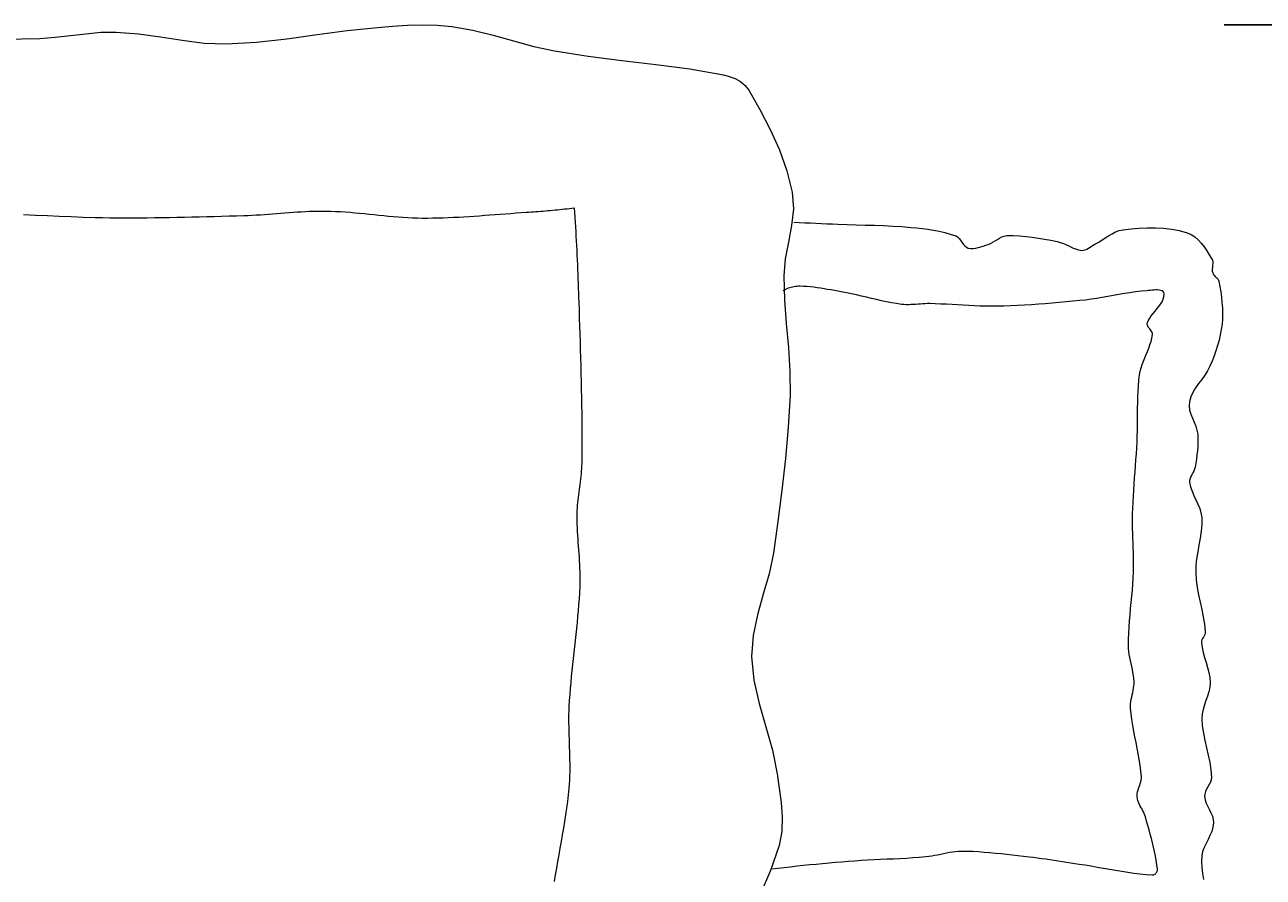
# Model space of a CAD drawing. Units: inches. Extents: x -15 to 423, y -713 to 71.
# Tile 22 of 24: x 311 to 364, y -137 to -101. Entities that reach past the tile are written whole.
import ezdxf

# ---------------------------------------------------------------- set-up
doc = ezdxf.new("R2010")
doc.units = ezdxf.units.IN
doc.header["$MEASUREMENT"] = 0
doc.layers.add('A-ANNO-DIMS', color=2, linetype='Continuous', lineweight=18)
doc.layers.add('A-FURN', color=9, linetype='Continuous', lineweight=13)
doc.styles.get("Standard").update_dxf_attribs({"font": 'arial.ttf'})
doc.dimstyles.get("Standard").update_dxf_attribs({"dimtxt": 0.18, "dimasz": 0.18, "dimexe": 0.18, "dimexo": 0.0625, "dimgap": 0.09, "dimtad": 0, "dimtih": 1, "dimtoh": 1, "dimdec": 0, "dimzin": 0, "dimdsep": 46, "dimlunit": 3, "dimtxsty": 'Standard', "dimcen": 0.09, "dimadec": 0, "dimazin": 0, "dimtfac": 1, "dimtdec": 0, "dimtofl": 0, "dimtmove": 0, "dimatfit": 3, "dimfxl": 1, "dimtolj": 1, "dimtzin": 0, "dimarcsym": 0})

# ---------------------------------------------------------------- blocks, each defined once
blk = doc.blocks.new('BED-DOUBLE')
for p, q in [((50.909, 70.114), (51.556, 70.189)), ((51.556, 70.189), (52.201, 70.268)), ((52.201, 70.268), (52.847, 70.326)), ((52.847, 70.326), (53.495, 70.339)), ((53.495, 70.339), (54.428, 70.266)), ((54.428, 70.266), (55.357, 70.134)), ((60.707, 70.052), (61.983, 70.229)), ((61.983, 70.229), (63.259, 70.403)), ((63.259, 70.403), (64.539, 70.536)), ((64.539, 70.536), (65.168, 70.585)), ((65.168, 70.585), (65.8, 70.625)), ((65.8, 70.625), (66.431, 70.645)), ((66.431, 70.645), (67.061, 70.633)), ((67.061, 70.633), (67.688, 70.576)), ((67.688, 70.576), (68.563, 70.418)), ((68.563, 70.418), (69.426, 70.201)), ((69.426, 70.201), (70.285, 69.959)), ((48.737, 70.043), (50.262, 70.068)), ((50.262, 70.068), (50.909, 70.114)), ((55.357, 70.134), (56.285, 69.988)), ((56.285, 69.988), (57.214, 69.874)), ((57.214, 69.874), (58.147, 69.837)), ((58.147, 69.837), (59.429, 69.908)), ((59.429, 69.908), (60.707, 70.052)), ((70.285, 69.959), (71.146, 69.727)), ((71.146, 69.727), (72.016, 69.538)), ((72.016, 69.538), (73.443, 69.316)), ((73.443, 69.316), (74.876, 69.137)), ((74.876, 69.137), (76.311, 68.967)), ((76.311, 68.967), (77.741, 68.775)), ((77.741, 68.775), (79.163, 68.528)), ((79.163, 68.528), (79.412, 68.464)), ((79.412, 68.464), (79.657, 68.368)), ((79.657, 68.368), (79.885, 68.24)), ((79.885, 68.24), (80.082, 68.078)), ((80.082, 68.078), (80.236, 67.88)), ((80.236, 67.88), (80.703, 67.06)), ((80.703, 67.06), (81.141, 66.219)), ((81.141, 66.219), (81.529, 65.356)), ((81.529, 65.356), (81.847, 64.47)), ((81.847, 64.47), (82.074, 63.56)), ((82.074, 63.56), (82.122, 62.86)), ((72.249, 62.834), (72.35, 62.845)), ((72.35, 62.845), (72.451, 62.855)), ((72.451, 62.855), (72.552, 62.866)), ((72.552, 62.866), (72.653, 62.877)), ((72.653, 62.877), (72.754, 62.888)), ((72.754, 62.888), (72.855, 62.9)), ((72.855, 62.9), (72.869, 62.701)), ((82.122, 62.86), (82.046, 62.156)), ((49.571, 62.62), (50.075, 62.595)), ((50.075, 62.595), (50.579, 62.572)), ((50.579, 62.572), (51.083, 62.55)), ((51.083, 62.55), (51.586, 62.53)), ((51.586, 62.53), (52.09, 62.513)), ((52.09, 62.513), (52.595, 62.499)), ((52.595, 62.499), (52.909, 62.492)), ((52.909, 62.492), (53.224, 62.487)), ((53.224, 62.487), (53.539, 62.483)), ((53.539, 62.483), (53.854, 62.481)), ((53.854, 62.481), (54.169, 62.481)), ((54.169, 62.481), (54.484, 62.482)), ((54.484, 62.482), (54.799, 62.484)), ((54.799, 62.484), (55.114, 62.488)), ((55.114, 62.488), (55.429, 62.492)), ((55.429, 62.492), (55.744, 62.497)), ((55.744, 62.497), (56.059, 62.504)), ((56.059, 62.504), (56.374, 62.511)), ((56.374, 62.511), (56.689, 62.518)), ((56.689, 62.518), (57.004, 62.526)), ((57.004, 62.526), (57.319, 62.535)), ((57.319, 62.535), (57.634, 62.543)), ((57.634, 62.543), (57.949, 62.552)), ((57.949, 62.552), (58.264, 62.561)), ((58.264, 62.561), (58.579, 62.57)), ((58.579, 62.57), (58.893, 62.579)), ((58.893, 62.579), (59.067, 62.585)), ((59.067, 62.585), (59.24, 62.592)), ((59.24, 62.592), (59.413, 62.602)), ((59.413, 62.602), (59.587, 62.612)), ((59.587, 62.612), (59.76, 62.624)), ((59.76, 62.624), (59.933, 62.637)), ((59.933, 62.637), (60.106, 62.65)), ((60.106, 62.65), (60.279, 62.663)), ((60.279, 62.663), (60.452, 62.677)), ((60.452, 62.677), (60.625, 62.691)), ((60.625, 62.691), (60.798, 62.704)), ((60.798, 62.704), (60.971, 62.717)), ((60.971, 62.717), (61.145, 62.729)), ((61.145, 62.729), (61.318, 62.739)), ((61.318, 62.739), (61.491, 62.749)), ((61.491, 62.749), (61.664, 62.756)), ((61.664, 62.756), (61.837, 62.762)), ((61.837, 62.762), (62.011, 62.766)), ((62.011, 62.766), (62.184, 62.768)), ((62.184, 62.768), (62.357, 62.767)), ((62.357, 62.767), (62.562, 62.762)), ((62.562, 62.762), (62.766, 62.754)), ((62.766, 62.754), (62.969, 62.743)), ((62.969, 62.743), (63.173, 62.73)), ((63.173, 62.73), (63.377, 62.714)), ((63.377, 62.714), (63.58, 62.696)), ((63.58, 62.696), (63.784, 62.677)), ((63.784, 62.677), (63.988, 62.657)), ((63.988, 62.657), (64.191, 62.637)), ((64.191, 62.637), (64.394, 62.616)), ((64.394, 62.616), (64.598, 62.595)), ((64.598, 62.595), (64.801, 62.574)), ((64.801, 62.574), (65.005, 62.555)), ((65.005, 62.555), (65.208, 62.537)), ((65.208, 62.537), (65.412, 62.52)), ((65.412, 62.52), (65.616, 62.505)), ((65.616, 62.505), (65.819, 62.493)), ((65.819, 62.493), (66.023, 62.483)), ((66.023, 62.483), (66.227, 62.476)), ((66.227, 62.476), (66.432, 62.473)), ((66.432, 62.473), (66.652, 62.473)), ((66.652, 62.473), (66.872, 62.475)), ((66.872, 62.475), (67.092, 62.479)), ((67.092, 62.479), (67.312, 62.486)), ((67.312, 62.486), (67.532, 62.494)), ((67.532, 62.494), (67.752, 62.503)), ((67.752, 62.503), (67.972, 62.514)), ((67.972, 62.514), (68.192, 62.527)), ((68.192, 62.527), (68.412, 62.54)), ((68.412, 62.54), (68.632, 62.555)), ((68.632, 62.555), (68.852, 62.57)), ((68.852, 62.57), (69.072, 62.586)), ((69.072, 62.586), (69.291, 62.602)), ((69.291, 62.602), (69.511, 62.619)), ((69.511, 62.619), (69.731, 62.636)), ((69.731, 62.636), (69.951, 62.652)), ((69.951, 62.652), (70.17, 62.669)), ((70.17, 62.669), (70.39, 62.685)), ((70.39, 62.685), (70.61, 62.701)), ((70.61, 62.701), (70.83, 62.716)), ((70.83, 62.716), (70.931, 62.723)), ((70.931, 62.723), (71.033, 62.73)), ((71.033, 62.73), (71.134, 62.737)), ((71.134, 62.737), (71.236, 62.745)), ((71.236, 62.745), (71.337, 62.753)), ((71.337, 62.753), (71.438, 62.761)), ((71.438, 62.761), (71.54, 62.769)), ((71.54, 62.769), (71.641, 62.778)), ((71.641, 62.778), (71.742, 62.787)), ((71.742, 62.787), (71.844, 62.796)), ((71.844, 62.796), (71.945, 62.805)), ((71.945, 62.805), (72.046, 62.814)), ((72.046, 62.814), (72.147, 62.824)), ((72.147, 62.824), (72.249, 62.834)), ((72.869, 62.701), (72.882, 62.501)), ((72.882, 62.501), (72.894, 62.302)), ((72.894, 62.302), (72.906, 62.103)), ((72.906, 62.103), (72.918, 61.903)), ((72.918, 61.903), (72.929, 61.704)), ((82.046, 62.156), (81.91, 61.449)), ((82.14, 62.295), (82.373, 62.284)), ((82.373, 62.284), (82.606, 62.273)), ((82.606, 62.273), (82.839, 62.263)), ((82.839, 62.263), (83.072, 62.252)), ((83.072, 62.252), (83.305, 62.242)), ((83.305, 62.242), (83.538, 62.231)), ((83.538, 62.231), (83.771, 62.221)), ((83.771, 62.221), (84.004, 62.21)), ((84.004, 62.21), (84.39, 62.196)), ((84.39, 62.196), (84.776, 62.185)), ((84.776, 62.185), (85.163, 62.175)), ((85.163, 62.175), (85.549, 62.165)), ((85.549, 62.165), (85.935, 62.152)), ((85.935, 62.152), (86.321, 62.134)), ((86.321, 62.134), (86.706, 62.11)), ((86.706, 62.11), (87.091, 62.077)), ((87.091, 62.077), (87.331, 62.053)), ((87.331, 62.053), (87.572, 62.025)), ((87.572, 62.025), (87.812, 61.994)), ((87.812, 61.994), (88.052, 61.957)), ((88.052, 61.957), (88.29, 61.912)), ((88.29, 61.912), (88.525, 61.859)), ((88.525, 61.859), (88.758, 61.795)), ((88.758, 61.795), (88.987, 61.72)), ((95.451, 61.723), (95.598, 61.81)), ((95.598, 61.81), (95.748, 61.884)), ((95.748, 61.884), (95.904, 61.941)), ((95.904, 61.941), (96.067, 61.975)), ((96.067, 61.975), (96.405, 62.013)), ((96.405, 62.013), (96.745, 62.042)), ((96.745, 62.042), (97.088, 62.058)), ((97.088, 62.058), (97.43, 62.06)), ((97.43, 62.06), (97.771, 62.042)), ((97.771, 62.042), (98.108, 62.004)), ((98.108, 62.004), (98.441, 61.941)), ((98.441, 61.941), (98.766, 61.851)), ((98.766, 61.851), (98.937, 61.777)), ((72.929, 61.704), (72.94, 61.505)), ((72.94, 61.505), (72.951, 61.305)), ((72.951, 61.305), (72.961, 61.106)), ((81.91, 61.449), (81.779, 60.741)), ((88.987, 61.72), (89.067, 61.676)), ((89.067, 61.676), (89.134, 61.612)), ((89.134, 61.612), (89.194, 61.536)), ((89.194, 61.536), (89.25, 61.453)), ((89.25, 61.453), (89.306, 61.371)), ((89.306, 61.371), (89.367, 61.298)), ((89.367, 61.298), (89.436, 61.239)), ((90.046, 61.25), (90.151, 61.285)), ((90.151, 61.285), (90.255, 61.321)), ((90.255, 61.321), (90.358, 61.356)), ((90.358, 61.356), (90.459, 61.397)), ((90.459, 61.397), (90.556, 61.45)), ((90.556, 61.45), (90.651, 61.509)), ((90.651, 61.509), (90.746, 61.57)), ((90.746, 61.57), (90.841, 61.627)), ((90.841, 61.627), (90.938, 61.675)), ((90.938, 61.675), (91.039, 61.71)), ((91.039, 61.71), (91.144, 61.726)), ((91.144, 61.726), (91.412, 61.729)), ((91.412, 61.729), (91.68, 61.719)), ((91.68, 61.719), (91.948, 61.697)), ((91.948, 61.697), (92.215, 61.665)), ((92.215, 61.665), (92.481, 61.626)), ((92.481, 61.626), (92.747, 61.58)), ((92.747, 61.58), (93.012, 61.531)), ((93.012, 61.531), (93.276, 61.479)), ((93.276, 61.479), (93.409, 61.444)), ((93.409, 61.444), (93.539, 61.395)), ((93.539, 61.395), (93.667, 61.337)), ((93.667, 61.337), (93.794, 61.275)), ((93.794, 61.275), (93.921, 61.216)), ((94.666, 61.238), (94.733, 61.282)), ((94.733, 61.282), (94.799, 61.325)), ((94.799, 61.325), (94.867, 61.363)), ((94.867, 61.363), (95.016, 61.444)), ((95.016, 61.444), (95.161, 61.535)), ((95.161, 61.535), (95.306, 61.63)), ((95.306, 61.63), (95.451, 61.723)), ((98.937, 61.777), (99.092, 61.674)), ((99.092, 61.674), (99.234, 61.548)), ((99.234, 61.548), (99.365, 61.405)), ((99.365, 61.405), (99.485, 61.248)), ((72.961, 61.106), (72.971, 60.906)), ((72.971, 60.906), (72.981, 60.707)), ((89.436, 61.239), (89.518, 61.202)), ((89.518, 61.202), (89.622, 61.184)), ((89.622, 61.184), (89.727, 61.183)), ((89.727, 61.183), (89.833, 61.195)), ((89.833, 61.195), (89.94, 61.219)), ((89.94, 61.219), (90.046, 61.25)), ((93.921, 61.216), (94.05, 61.164)), ((94.05, 61.164), (94.181, 61.125)), ((94.181, 61.125), (94.316, 61.104)), ((94.316, 61.104), (94.391, 61.107)), ((94.391, 61.107), (94.462, 61.126)), ((94.462, 61.126), (94.531, 61.156)), ((94.531, 61.156), (94.599, 61.194)), ((94.599, 61.194), (94.666, 61.238)), ((99.485, 61.248), (99.598, 61.085)), ((99.598, 61.085), (99.705, 60.919)), ((99.705, 60.919), (99.808, 60.757)), ((99.808, 60.757), (99.838, 60.69)), ((72.981, 60.707), (72.99, 60.507)), ((72.99, 60.507), (72.999, 60.308)), ((72.999, 60.308), (73.007, 60.108)), ((81.779, 60.741), (81.716, 60.031)), ((99.839, 60.384), (99.834, 60.305)), ((99.834, 60.305), (99.836, 60.227)), ((99.836, 60.227), (99.852, 60.153)), ((99.838, 60.69), (99.852, 60.618)), ((99.847, 60.463), (99.839, 60.384)), ((99.853, 60.542), (99.847, 60.463)), ((99.852, 60.618), (99.853, 60.542)), ((73.007, 60.108), (73.015, 59.909)), ((73.015, 59.909), (73.023, 59.709)), ((73.023, 59.709), (73.03, 59.51)), ((81.716, 60.031), (81.743, 59.019)), ((99.852, 60.153), (99.875, 60.104)), ((99.875, 60.104), (99.908, 60.059)), ((99.908, 60.059), (99.948, 60.017)), ((99.948, 60.017), (99.99, 59.977)), ((99.99, 59.977), (100.032, 59.936)), ((100.032, 59.936), (100.069, 59.894)), ((100.069, 59.894), (100.098, 59.848)), ((100.098, 59.848), (100.115, 59.797)), ((100.115, 59.797), (100.154, 59.573)), ((73.03, 59.51), (73.037, 59.31)), ((73.037, 59.31), (73.044, 59.111)), ((81.735, 59.422), (81.681, 59.391)), ((81.791, 59.451), (81.735, 59.422)), ((81.849, 59.477), (81.791, 59.451)), ((81.908, 59.5), (81.849, 59.477)), ((81.968, 59.521), (81.908, 59.5)), ((82.029, 59.539), (81.968, 59.521)), ((82.091, 59.554), (82.029, 59.539)), ((82.153, 59.567), (82.091, 59.554)), ((82.216, 59.576), (82.153, 59.567)), ((82.279, 59.583), (82.216, 59.576)), ((82.342, 59.586), (82.279, 59.583)), ((82.405, 59.587), (82.342, 59.586)), ((82.551, 59.582), (82.405, 59.587)), ((82.697, 59.573), (82.551, 59.582)), ((82.843, 59.56), (82.697, 59.573)), ((82.989, 59.544), (82.843, 59.56)), ((83.134, 59.525), (82.989, 59.544)), ((83.28, 59.503), (83.134, 59.525)), ((83.425, 59.48), (83.28, 59.503)), ((83.57, 59.455), (83.425, 59.48)), ((83.715, 59.429), (83.57, 59.455)), ((83.859, 59.403), (83.715, 59.429)), ((84.004, 59.376), (83.859, 59.403)), ((84.148, 59.35), (84.004, 59.376)), ((84.362, 59.31), (84.148, 59.35)), ((84.574, 59.266), (84.362, 59.31)), ((84.787, 59.219), (84.574, 59.266)), ((84.999, 59.171), (84.787, 59.219)), ((95.649, 59.195), (95.414, 59.154)), ((95.884, 59.236), (95.649, 59.195)), ((96.119, 59.275), (95.884, 59.236)), ((96.354, 59.312), (96.119, 59.275)), ((96.59, 59.345), (96.354, 59.312)), ((96.826, 59.373), (96.59, 59.345)), ((97.064, 59.395), (96.826, 59.373)), ((97.13, 59.401), (97.064, 59.395)), ((97.204, 59.409), (97.13, 59.401)), ((97.283, 59.417), (97.204, 59.409)), ((97.364, 59.424), (97.283, 59.417)), ((97.444, 59.429), (97.364, 59.424)), ((97.523, 59.429), (97.444, 59.429)), ((97.596, 59.423), (97.523, 59.429)), ((97.661, 59.411), (97.596, 59.423)), ((97.717, 59.389), (97.661, 59.411)), ((97.76, 59.358), (97.717, 59.389)), ((97.788, 59.316), (97.76, 59.358)), ((97.799, 59.261), (97.788, 59.316)), ((97.789, 59.144), (97.799, 59.261)), ((100.154, 59.573), (100.19, 59.348)), ((100.19, 59.348), (100.221, 59.121)), ((73.044, 59.111), (73.05, 58.911)), ((73.05, 58.911), (73.06, 58.576)), ((81.743, 59.019), (81.82, 58.007)), ((85.21, 59.121), (84.999, 59.171)), ((85.422, 59.072), (85.21, 59.121)), ((85.634, 59.023), (85.422, 59.072)), ((85.846, 58.976), (85.634, 59.023)), ((86.059, 58.931), (85.846, 58.976)), ((86.272, 58.89), (86.059, 58.931)), ((86.486, 58.853), (86.272, 58.89)), ((86.701, 58.821), (86.486, 58.853)), ((86.799, 58.811), (86.701, 58.821)), ((86.897, 58.806), (86.799, 58.811)), ((86.996, 58.805), (86.897, 58.806)), ((87.095, 58.808), (86.996, 58.805)), ((87.193, 58.813), (87.095, 58.808)), ((87.292, 58.819), (87.193, 58.813)), ((87.392, 58.827), (87.292, 58.819)), ((87.491, 58.835), (87.392, 58.827)), ((87.59, 58.842), (87.491, 58.835)), ((87.689, 58.848), (87.59, 58.842)), ((87.788, 58.851), (87.689, 58.848)), ((87.887, 58.851), (87.788, 58.851)), ((88.123, 58.845), (87.887, 58.851)), ((88.359, 58.835), (88.123, 58.845)), ((88.596, 58.824), (88.359, 58.835)), ((88.832, 58.81), (88.596, 58.824)), ((89.068, 58.797), (88.832, 58.81)), ((89.304, 58.783), (89.068, 58.797)), ((89.54, 58.77), (89.304, 58.783)), ((89.777, 58.758), (89.54, 58.77)), ((90.013, 58.749), (89.777, 58.758)), ((90.249, 58.743), (90.013, 58.749)), ((90.485, 58.741), (90.249, 58.743)), ((90.722, 58.743), (90.485, 58.741)), ((91.015, 58.75), (90.722, 58.743)), ((91.308, 58.76), (91.015, 58.75)), ((91.602, 58.773), (91.308, 58.76)), ((91.895, 58.788), (91.602, 58.773)), ((92.188, 58.805), (91.895, 58.788)), ((92.481, 58.824), (92.188, 58.805)), ((92.774, 58.846), (92.481, 58.824)), ((93.066, 58.869), (92.774, 58.846)), ((93.359, 58.894), (93.066, 58.869)), ((93.651, 58.921), (93.359, 58.894)), ((93.943, 58.949), (93.651, 58.921)), ((94.235, 58.978), (93.943, 58.949)), ((94.472, 59.005), (94.235, 58.978)), ((94.708, 59.038), (94.472, 59.005)), ((94.944, 59.074), (94.708, 59.038)), ((95.179, 59.113), (94.944, 59.074)), ((95.414, 59.154), (95.179, 59.113)), ((97.496, 58.631), (97.575, 58.728)), ((97.575, 58.728), (97.648, 58.827)), ((97.648, 58.827), (97.71, 58.929)), ((97.71, 58.929), (97.758, 59.034)), ((97.758, 59.034), (97.789, 59.144)), ((100.221, 59.121), (100.245, 58.894)), ((100.245, 58.894), (100.261, 58.667)), ((100.261, 58.667), (100.267, 58.439)), ((73.06, 58.576), (73.07, 58.24)), ((73.07, 58.24), (73.081, 57.905)), ((97.088, 58.015), (97.13, 58.127)), ((97.13, 58.127), (97.187, 58.233)), ((97.187, 58.233), (97.256, 58.336)), ((97.256, 58.336), (97.333, 58.436)), ((97.333, 58.436), (97.414, 58.534)), ((97.414, 58.534), (97.496, 58.631)), ((100.263, 58.213), (100.246, 57.986)), ((100.267, 58.439), (100.263, 58.213)), ((73.081, 57.905), (73.091, 57.57)), ((81.82, 58.007), (81.91, 56.995)), ((97.083, 57.974), (97.088, 58.015)), ((97.09, 57.934), (97.083, 57.974)), ((97.106, 57.895), (97.09, 57.934)), ((97.13, 57.856), (97.106, 57.895)), ((97.159, 57.818), (97.13, 57.856)), ((97.191, 57.78), (97.159, 57.818)), ((97.223, 57.743), (97.191, 57.78)), ((97.253, 57.704), (97.223, 57.743)), ((97.28, 57.666), (97.253, 57.704)), ((97.299, 57.626), (97.28, 57.666)), ((97.31, 57.585), (97.299, 57.626)), ((100.215, 57.758), (100.172, 57.53)), ((100.246, 57.986), (100.215, 57.758)), ((73.091, 57.57), (73.101, 57.234)), ((73.101, 57.234), (73.111, 56.899)), ((97.148, 56.972), (97.199, 57.112)), ((97.199, 57.112), (97.245, 57.254)), ((97.245, 57.254), (97.282, 57.397)), ((97.282, 57.397), (97.31, 57.543)), ((97.31, 57.543), (97.31, 57.585)), ((100.056, 57.082), (99.985, 56.861)), ((100.119, 57.305), (100.056, 57.082)), ((100.172, 57.53), (100.119, 57.305)), ((73.111, 56.899), (73.121, 56.563)), ((73.121, 56.563), (73.13, 56.228)), ((81.91, 56.995), (81.976, 55.984)), ((96.923, 56.417), (96.978, 56.556)), ((96.978, 56.556), (97.036, 56.695)), ((97.036, 56.695), (97.093, 56.833)), ((97.093, 56.833), (97.148, 56.972)), ((99.907, 56.642), (99.824, 56.425)), ((99.985, 56.861), (99.907, 56.642)), ((73.13, 56.228), (73.139, 55.893)), ((96.79, 55.992), (96.827, 56.135)), ((96.827, 56.135), (96.872, 56.276)), ((96.872, 56.276), (96.923, 56.417)), ((99.736, 56.211), (99.638, 56.015)), ((99.824, 56.425), (99.736, 56.211)), ((73.139, 55.893), (73.147, 55.557)), ((73.147, 55.557), (73.154, 55.222)), ((81.976, 55.984), (81.981, 54.972)), ((96.712, 55.377), (96.734, 55.611)), ((96.734, 55.611), (96.763, 55.846)), ((96.763, 55.846), (96.79, 55.992)), ((99.388, 55.647), (99.254, 55.467)), ((99.519, 55.828), (99.388, 55.647)), ((99.638, 56.015), (99.519, 55.828)), ((73.154, 55.222), (73.161, 54.886)), ((96.686, 54.905), (96.696, 55.141)), ((96.696, 55.141), (96.712, 55.377)), ((99.012, 55.1), (98.921, 54.904)), ((99.125, 55.286), (99.012, 55.1)), ((99.254, 55.467), (99.125, 55.286)), ((73.161, 54.886), (73.167, 54.551)), ((73.167, 54.551), (73.172, 54.215)), ((81.981, 54.972), (81.907, 53.633)), ((96.677, 54.432), (96.68, 54.668)), ((96.68, 54.668), (96.686, 54.905)), ((98.864, 54.697), (98.853, 54.524)), ((98.853, 54.524), (98.878, 54.353)), ((98.921, 54.904), (98.864, 54.697)), ((73.172, 54.215), (73.176, 53.88)), ((96.674, 53.721), (96.675, 53.958)), ((96.675, 54.195), (96.677, 54.432)), ((96.675, 53.958), (96.675, 54.195)), ((98.878, 54.353), (98.928, 54.183)), ((98.928, 54.183), (98.994, 54.014)), ((98.994, 54.014), (99.066, 53.845)), ((73.176, 53.88), (73.179, 53.545)), ((73.179, 53.545), (73.181, 53.209)), ((81.907, 53.633), (81.79, 52.296)), ((96.665, 53.247), (96.671, 53.484)), ((96.671, 53.484), (96.674, 53.721)), ((99.066, 53.845), (99.134, 53.674)), ((99.134, 53.674), (99.188, 53.502)), ((99.188, 53.502), (99.219, 53.328)), ((73.181, 53.209), (73.181, 52.874)), ((96.641, 52.755), (96.656, 53.011)), ((96.656, 53.011), (96.665, 53.247)), ((99.219, 53.328), (99.229, 53.153)), ((99.23, 52.978), (99.222, 52.803)), ((99.229, 53.153), (99.23, 52.978)), ((73.18, 52.538), (73.178, 52.203)), ((73.181, 52.874), (73.18, 52.538)), ((96.608, 52.244), (96.625, 52.5)), ((96.625, 52.5), (96.641, 52.755)), ((99.187, 52.453), (99.163, 52.278)), ((99.207, 52.628), (99.187, 52.453)), ((99.222, 52.803), (99.207, 52.628)), ((73.164, 51.87), (73.155, 51.76)), ((73.171, 51.981), (73.164, 51.87)), ((73.176, 52.092), (73.171, 51.981)), ((73.178, 52.203), (73.176, 52.092)), ((81.79, 52.296), (81.64, 50.963)), ((96.57, 51.734), (96.589, 51.989)), ((96.589, 51.989), (96.608, 52.244)), ((99.085, 51.849), (99.051, 51.769)), ((99.107, 51.931), (99.085, 51.849)), ((99.136, 52.104), (99.107, 51.931)), ((99.163, 52.278), (99.136, 52.104)), ((73.105, 51.318), (73.09, 51.208)), ((73.119, 51.428), (73.105, 51.318)), ((73.132, 51.539), (73.119, 51.428)), ((73.144, 51.649), (73.132, 51.539)), ((73.155, 51.76), (73.144, 51.649)), ((96.533, 51.223), (96.551, 51.478)), ((96.551, 51.478), (96.57, 51.734)), ((98.896, 51.458), (98.878, 51.378)), ((98.878, 51.378), (98.878, 51.295)), ((98.928, 51.536), (98.896, 51.458)), ((98.968, 51.614), (98.928, 51.536)), ((99.01, 51.691), (98.968, 51.614)), ((99.051, 51.769), (99.01, 51.691)), ((73.046, 50.877), (73.032, 50.767)), ((73.061, 50.987), (73.046, 50.877)), ((73.076, 51.098), (73.061, 50.987)), ((73.09, 51.208), (73.076, 51.098)), ((81.64, 50.963), (81.466, 49.632)), ((96.499, 50.712), (96.515, 50.968)), ((96.515, 50.968), (96.533, 51.223)), ((98.878, 51.295), (98.918, 51.103)), ((98.918, 51.103), (98.981, 50.917)), ((98.981, 50.917), (99.059, 50.733)), ((72.985, 50.325), (72.977, 50.214)), ((72.995, 50.435), (72.985, 50.325)), ((73.006, 50.546), (72.995, 50.435)), ((73.018, 50.656), (73.006, 50.546)), ((73.032, 50.767), (73.018, 50.656)), ((96.473, 50.201), (96.485, 50.456)), ((96.485, 50.456), (96.499, 50.712)), ((99.059, 50.733), (99.144, 50.552)), ((99.144, 50.552), (99.228, 50.37)), ((99.228, 50.37), (99.301, 50.186)), ((72.969, 49.992), (72.967, 49.837)), ((72.967, 49.837), (72.969, 49.681)), ((72.972, 50.103), (72.969, 49.992)), ((72.977, 50.214), (72.972, 50.103)), ((96.461, 49.743), (96.464, 49.945)), ((96.464, 49.945), (96.473, 50.201)), ((99.301, 50.186), (99.357, 49.999)), ((99.357, 49.999), (99.386, 49.806)), ((99.386, 49.806), (99.389, 49.514)), ((72.969, 49.681), (72.973, 49.525)), ((72.973, 49.525), (72.978, 49.37)), ((72.978, 49.37), (72.986, 49.214)), ((81.466, 49.632), (81.275, 48.303)), ((96.461, 49.54), (96.461, 49.743)), ((96.464, 49.337), (96.461, 49.54)), ((96.47, 49.135), (96.464, 49.337)), ((99.365, 49.224), (99.323, 48.933)), ((99.389, 49.514), (99.365, 49.224)), ((72.986, 49.214), (72.995, 49.058)), ((72.995, 49.058), (73.004, 48.903)), ((73.004, 48.903), (73.015, 48.747)), ((73.015, 48.747), (73.026, 48.591)), ((96.477, 48.932), (96.47, 49.135)), ((96.484, 48.73), (96.477, 48.932)), ((96.492, 48.527), (96.484, 48.73)), ((99.323, 48.933), (99.271, 48.643)), ((73.026, 48.591), (73.037, 48.436)), ((73.037, 48.436), (73.048, 48.28)), ((73.048, 48.28), (73.059, 48.125)), ((81.275, 48.303), (81.093, 47.426)), ((96.499, 48.325), (96.492, 48.527)), ((96.504, 48.122), (96.499, 48.325)), ((99.217, 48.353), (99.171, 48.063)), ((99.271, 48.643), (99.217, 48.353)), ((73.059, 48.125), (73.068, 47.969)), ((73.068, 47.969), (73.077, 47.813)), ((73.077, 47.813), (73.084, 47.658)), ((73.084, 47.658), (73.09, 47.502)), ((96.502, 47.515), (96.506, 47.717)), ((96.507, 47.92), (96.504, 48.122)), ((96.506, 47.717), (96.507, 47.92)), ((99.141, 47.772), (99.135, 47.48)), ((99.171, 48.063), (99.141, 47.772)), ((73.09, 47.502), (73.093, 47.347)), ((73.094, 47.191), (73.092, 47.035)), ((73.093, 47.347), (73.094, 47.191)), ((81.093, 47.426), (80.849, 46.558)), ((96.475, 46.994), (96.491, 47.254)), ((96.491, 47.254), (96.502, 47.515)), ((99.135, 47.48), (99.157, 47.165)), ((99.157, 47.165), (99.2, 46.852)), ((73.075, 46.626), (73.06, 46.373)), ((73.087, 46.88), (73.075, 46.626)), ((73.092, 47.035), (73.087, 46.88)), ((96.432, 46.473), (96.455, 46.733)), ((96.455, 46.733), (96.475, 46.994)), ((99.2, 46.852), (99.257, 46.541)), ((73.042, 46.119), (73.022, 45.866)), ((73.06, 46.373), (73.042, 46.119)), ((80.849, 46.558), (80.603, 45.691)), ((96.382, 45.953), (96.407, 46.213)), ((96.407, 46.213), (96.432, 46.473)), ((99.257, 46.541), (99.322, 46.23)), ((99.322, 46.23), (99.389, 45.92)), ((73, 45.613), (72.976, 45.36)), ((73.022, 45.866), (73, 45.613)), ((80.603, 45.691), (80.417, 44.818)), ((96.336, 45.433), (96.358, 45.693)), ((96.358, 45.693), (96.382, 45.953)), ((99.389, 45.92), (99.452, 45.609)), ((99.452, 45.609), (99.505, 45.296)), ((72.95, 45.107), (72.924, 44.854)), ((72.976, 45.36), (72.95, 45.107)), ((96.302, 44.912), (96.317, 45.173)), ((96.317, 45.173), (96.336, 45.433)), ((99.505, 45.296), (99.54, 44.982)), ((72.897, 44.601), (72.869, 44.349)), ((72.924, 44.854), (72.897, 44.601)), ((80.417, 44.818), (80.352, 43.933)), ((96.29, 44.391), (96.293, 44.652)), ((96.293, 44.652), (96.302, 44.912)), ((99.377, 44.58), (99.374, 44.52)), ((99.374, 44.52), (99.405, 44.305)), ((99.395, 44.638), (99.377, 44.58)), ((99.423, 44.695), (99.395, 44.638)), ((99.456, 44.751), (99.423, 44.695)), ((99.489, 44.807), (99.456, 44.751)), ((99.518, 44.864), (99.489, 44.807)), ((99.536, 44.922), (99.518, 44.864)), ((99.54, 44.982), (99.536, 44.922)), ((72.841, 44.096), (72.813, 43.843)), ((72.869, 44.349), (72.841, 44.096)), ((96.295, 44.263), (96.29, 44.391)), ((96.307, 44.136), (96.295, 44.263)), ((96.325, 44.009), (96.307, 44.136)), ((96.348, 43.882), (96.325, 44.009)), ((99.405, 44.305), (99.453, 44.092)), ((99.453, 44.092), (99.512, 43.881)), ((72.785, 43.591), (72.759, 43.338)), ((72.813, 43.843), (72.785, 43.591)), ((80.352, 43.933), (80.453, 42.928)), ((96.374, 43.756), (96.348, 43.882)), ((96.402, 43.63), (96.374, 43.756)), ((96.43, 43.504), (96.402, 43.63)), ((96.457, 43.378), (96.43, 43.504)), ((99.512, 43.881), (99.576, 43.671)), ((99.576, 43.671), (99.637, 43.46)), ((72.733, 43.085), (72.709, 42.832)), ((72.759, 43.338), (72.733, 43.085)), ((96.481, 43.251), (96.457, 43.378)), ((96.502, 43.124), (96.481, 43.251)), ((96.517, 42.997), (96.502, 43.124)), ((96.525, 42.869), (96.517, 42.997)), ((99.637, 43.46), (99.689, 43.249)), ((99.689, 43.249), (99.726, 43.036)), ((99.726, 43.036), (99.74, 42.82)), ((72.687, 42.579), (72.667, 42.325)), ((72.709, 42.832), (72.687, 42.579)), ((80.453, 42.928), (80.676, 41.938)), ((96.468, 42.4), (96.487, 42.494)), ((96.487, 42.494), (96.504, 42.587)), ((96.504, 42.587), (96.517, 42.681)), ((96.517, 42.681), (96.525, 42.775)), ((96.525, 42.775), (96.525, 42.869)), ((99.686, 42.439), (99.63, 42.252)), ((99.726, 42.628), (99.686, 42.439)), ((99.74, 42.82), (99.726, 42.628)), ((72.649, 42.072), (72.634, 41.818)), ((72.667, 42.325), (72.649, 42.072)), ((80.676, 41.938), (80.958, 40.954)), ((96.378, 41.839), (96.383, 41.933)), ((96.383, 41.933), (96.393, 42.027)), ((96.393, 42.027), (96.409, 42.12)), ((96.409, 42.12), (96.427, 42.214)), ((96.427, 42.214), (96.447, 42.307)), ((96.447, 42.307), (96.468, 42.4)), ((99.565, 42.066), (99.5, 41.88)), ((99.63, 42.252), (99.565, 42.066)), ((72.621, 41.473), (72.619, 41.3)), ((72.626, 41.646), (72.621, 41.473)), ((72.634, 41.818), (72.626, 41.646)), ((96.381, 41.746), (96.378, 41.839)), ((96.405, 41.502), (96.381, 41.746)), ((96.436, 41.259), (96.405, 41.502)), ((99.406, 41.504), (99.393, 41.313)), ((99.444, 41.693), (99.406, 41.504)), ((99.5, 41.88), (99.444, 41.693)), ((72.619, 41.3), (72.62, 41.127)), ((72.62, 41.127), (72.622, 40.954)), ((72.622, 40.954), (72.625, 40.78)), ((80.958, 40.954), (81.233, 39.968)), ((96.474, 41.016), (96.436, 41.259)), ((96.516, 40.775), (96.474, 41.016)), ((99.393, 41.313), (99.412, 40.998)), ((99.412, 40.998), (99.457, 40.685)), ((72.625, 40.78), (72.63, 40.607)), ((72.63, 40.607), (72.636, 40.434)), ((72.636, 40.434), (72.642, 40.261)), ((96.562, 40.533), (96.516, 40.775)), ((96.609, 40.292), (96.562, 40.533)), ((99.457, 40.685), (99.519, 40.374)), ((99.519, 40.374), (99.589, 40.064)), ((72.642, 40.261), (72.648, 40.088)), ((72.648, 40.088), (72.654, 39.914)), ((72.654, 39.914), (72.659, 39.741)), ((81.233, 39.968), (81.436, 38.971)), ((96.656, 40.051), (96.609, 40.292)), ((96.702, 39.81), (96.656, 40.051)), ((96.744, 39.568), (96.702, 39.81)), ((99.589, 40.064), (99.661, 39.753)), ((72.659, 39.741), (72.662, 39.568)), ((72.662, 39.568), (72.665, 39.395)), ((72.665, 39.395), (72.665, 39.222)), ((96.782, 39.326), (96.744, 39.568)), ((96.812, 39.083), (96.782, 39.326)), ((99.661, 39.753), (99.724, 39.442)), ((99.724, 39.442), (99.773, 39.13)), ((72.659, 38.877), (72.652, 38.704)), ((72.664, 39.049), (72.659, 38.877)), ((72.665, 39.222), (72.664, 39.049)), ((81.436, 38.971), (81.528, 38.364)), ((96.835, 38.839), (96.812, 39.083)), ((96.827, 38.695), (96.836, 38.767)), ((96.836, 38.767), (96.835, 38.839)), ((99.773, 39.13), (99.798, 38.815)), ((99.798, 38.815), (99.788, 38.71)), ((72.627, 38.359), (72.598, 38.076)), ((72.641, 38.531), (72.627, 38.359)), ((72.652, 38.704), (72.641, 38.531)), ((81.528, 38.364), (81.611, 37.75)), ((96.677, 38.202), (96.696, 38.272)), ((96.696, 38.272), (96.719, 38.343)), ((96.719, 38.343), (96.744, 38.413)), ((96.744, 38.413), (96.769, 38.483)), ((96.769, 38.483), (96.792, 38.554)), ((96.792, 38.554), (96.812, 38.624)), ((96.812, 38.624), (96.827, 38.695)), ((99.596, 38.312), (99.548, 38.213)), ((99.651, 38.41), (99.596, 38.312)), ((99.707, 38.509), (99.651, 38.41)), ((99.755, 38.608), (99.707, 38.509)), ((99.788, 38.71), (99.755, 38.608)), ((72.565, 37.793), (72.528, 37.51)), ((72.598, 38.076), (72.565, 37.793)), ((81.611, 37.75), (81.655, 37.136)), ((96.657, 38.06), (96.663, 38.131)), ((96.659, 37.988), (96.657, 38.06)), ((96.671, 37.913), (96.659, 37.988)), ((96.663, 38.131), (96.677, 38.202)), ((96.69, 37.84), (96.671, 37.913)), ((96.715, 37.769), (96.69, 37.84)), ((96.745, 37.699), (96.715, 37.769)), ((99.516, 38.111), (99.507, 38.006)), ((99.507, 38.006), (99.529, 37.861)), ((99.548, 38.213), (99.516, 38.111)), ((99.529, 37.861), (99.576, 37.721)), ((99.576, 37.721), (99.64, 37.583)), ((72.488, 37.228), (72.445, 36.947)), ((72.528, 37.51), (72.488, 37.228)), ((96.778, 37.63), (96.745, 37.699)), ((96.814, 37.562), (96.778, 37.63)), ((96.851, 37.494), (96.814, 37.562)), ((96.887, 37.425), (96.851, 37.494)), ((96.923, 37.357), (96.887, 37.425)), ((96.955, 37.287), (96.923, 37.357)), ((96.984, 37.216), (96.955, 37.287)), ((97.008, 37.144), (96.984, 37.216)), ((99.64, 37.583), (99.711, 37.447)), ((99.711, 37.447), (99.78, 37.311)), ((99.78, 37.311), (99.838, 37.174)), ((72.399, 36.665), (72.352, 36.384)), ((72.445, 36.947), (72.399, 36.665)), ((81.655, 37.136), (81.634, 36.529)), ((97.059, 36.962), (97.008, 37.144)), ((97.11, 36.78), (97.059, 36.962)), ((97.161, 36.597), (97.11, 36.78)), ((99.862, 36.708), (99.809, 36.534)), ((99.838, 37.174), (99.877, 37.034)), ((99.888, 36.889), (99.862, 36.708)), ((99.877, 37.034), (99.888, 36.889)), ((72.352, 36.384), (72.303, 36.103)), ((81.634, 36.529), (81.518, 35.937)), ((97.211, 36.414), (97.161, 36.597)), ((97.26, 36.231), (97.211, 36.414)), ((97.306, 36.048), (97.26, 36.231)), ((99.654, 36.194), (99.569, 36.025)), ((99.737, 36.363), (99.654, 36.194)), ((99.809, 36.534), (99.737, 36.363)), ((72.254, 35.822), (72.204, 35.541)), ((72.303, 36.103), (72.254, 35.822)), ((81.518, 35.937), (81.158, 34.884)), ((88.476, 35.6), (88.602, 35.626)), ((88.602, 35.626), (88.728, 35.65)), ((88.728, 35.65), (88.855, 35.67)), ((88.855, 35.67), (88.982, 35.686)), ((88.982, 35.686), (89.109, 35.697)), ((89.109, 35.697), (89.237, 35.7)), ((89.237, 35.7), (89.476, 35.697)), ((89.476, 35.697), (89.714, 35.689)), ((89.714, 35.689), (89.952, 35.676)), ((89.952, 35.676), (90.19, 35.659)), ((90.19, 35.659), (90.428, 35.639)), ((90.428, 35.639), (90.665, 35.617)), ((90.665, 35.617), (90.903, 35.592)), ((97.35, 35.864), (97.306, 36.048)), ((97.391, 35.68), (97.35, 35.864)), ((97.429, 35.494), (97.391, 35.68)), ((99.427, 35.681), (99.387, 35.502)), ((99.49, 35.855), (99.427, 35.681)), ((99.569, 36.025), (99.49, 35.855)), ((72.153, 35.261), (72.103, 34.98)), ((72.204, 35.541), (72.153, 35.261)), ((82.275, 35.069), (82.546, 35.098)), ((82.546, 35.098), (82.818, 35.125)), ((82.818, 35.125), (83.089, 35.152)), ((83.089, 35.152), (83.36, 35.178)), ((83.36, 35.178), (83.631, 35.203)), ((83.631, 35.203), (83.903, 35.227)), ((83.903, 35.227), (84.174, 35.251)), ((84.174, 35.251), (84.446, 35.273)), ((84.446, 35.273), (84.718, 35.293)), ((84.718, 35.293), (84.991, 35.311)), ((84.991, 35.311), (85.263, 35.326)), ((85.263, 35.326), (85.536, 35.34)), ((85.536, 35.34), (85.809, 35.353)), ((85.809, 35.353), (86.081, 35.365)), ((86.081, 35.365), (86.354, 35.378)), ((86.354, 35.378), (86.627, 35.392)), ((86.627, 35.392), (86.899, 35.406)), ((86.899, 35.406), (87.172, 35.423)), ((87.172, 35.423), (87.444, 35.443)), ((87.444, 35.443), (87.716, 35.465)), ((87.716, 35.465), (87.843, 35.479)), ((87.843, 35.479), (87.97, 35.499)), ((87.97, 35.499), (88.097, 35.521)), ((88.097, 35.521), (88.223, 35.547)), ((88.223, 35.547), (88.35, 35.573)), ((88.35, 35.573), (88.476, 35.6)), ((90.903, 35.592), (91.14, 35.565)), ((91.14, 35.565), (91.377, 35.538)), ((91.377, 35.538), (91.614, 35.51)), ((91.614, 35.51), (91.851, 35.483)), ((91.851, 35.483), (92.088, 35.456)), ((92.088, 35.456), (92.265, 35.436)), ((92.265, 35.436), (92.441, 35.414)), ((92.441, 35.414), (92.617, 35.39)), ((92.617, 35.39), (92.793, 35.365)), ((92.793, 35.365), (92.969, 35.34)), ((92.969, 35.34), (93.145, 35.314)), ((93.145, 35.314), (93.321, 35.287)), ((93.321, 35.287), (93.497, 35.259)), ((93.497, 35.259), (93.672, 35.232)), ((93.672, 35.232), (93.848, 35.205)), ((93.848, 35.205), (94.024, 35.178)), ((94.024, 35.178), (94.199, 35.152)), ((94.199, 35.152), (94.458, 35.112)), ((94.458, 35.112), (94.715, 35.069)), ((97.463, 35.309), (97.429, 35.494)), ((97.493, 35.122), (97.463, 35.309)), ((97.518, 34.935), (97.493, 35.122)), ((99.387, 35.502), (99.374, 35.255)), ((99.374, 35.255), (99.391, 35.004)), ((72.054, 34.699), (72.006, 34.418)), ((72.103, 34.98), (72.054, 34.699)), ((81.158, 34.884), (80.717, 33.859)), ((81.192, 34.944), (81.463, 34.976)), ((81.463, 34.976), (81.734, 35.008)), ((81.734, 35.008), (82.005, 35.039)), ((82.005, 35.039), (82.275, 35.069)), ((94.715, 35.069), (94.973, 35.025)), ((94.973, 35.025), (95.23, 34.979)), ((95.23, 34.979), (95.488, 34.933)), ((95.488, 34.933), (95.745, 34.888)), ((95.745, 34.888), (96.003, 34.845)), ((96.003, 34.845), (96.261, 34.805)), ((96.261, 34.805), (96.519, 34.768)), ((96.519, 34.768), (96.778, 34.735)), ((96.778, 34.735), (97.038, 34.708)), ((97.038, 34.708), (97.298, 34.688)), ((97.298, 34.688), (97.325, 34.689)), ((97.325, 34.689), (97.353, 34.696)), ((97.353, 34.696), (97.38, 34.708)), ((97.38, 34.708), (97.406, 34.724)), ((97.406, 34.724), (97.431, 34.744)), ((97.431, 34.744), (97.454, 34.768)), ((97.454, 34.768), (97.474, 34.793)), ((97.474, 34.793), (97.491, 34.821)), ((97.491, 34.821), (97.504, 34.849)), ((97.504, 34.849), (97.513, 34.878)), ((97.513, 34.878), (97.518, 34.907)), ((97.518, 34.907), (97.518, 34.935)), ((99.391, 35.004), (99.427, 34.751)), ((99.427, 34.751), (99.468, 34.498))]:
    blk.add_line(p, q)
blk = doc.blocks.new('*D32')
at = {"layer": 'A-ANNO-DIMS', "color": 0, "lineweight": -2, "transparency": 16777216}
for p, q in [((361.968, -101.283), (377.126, -101.283)), ((376.946, -101.463), (376.946, -136.422)), ((376.946, -171.748), (376.946, -136.788)), ((361.968, -171.928), (377.126, -171.928))]:
    blk.add_line(p, q, dxfattribs=at)
at = {"layer": 'A-ANNO-DIMS', "color": 0, "transparency": 16777216}
for points in [[(376.916, -101.463), (376.976, -101.463), (376.946, -101.283)], [(376.916, -171.748), (376.976, -171.748), (376.946, -171.928)]]:
    blk.add_solid(points, dxfattribs=at)
at = {"layer": 'Defpoints', "color": 0, "transparency": 16777216}
for p in [(361.906, -101.283), (376.946, -101.283), (361.906, -171.928)]:
    blk.add_point(p, dxfattribs=at)
at = {"layer": 'A-ANNO-DIMS', "color": 0, "transparency": 16777216, "insert": (376.946, -136.605), "char_height": 0.18, "attachment_point": 5}
blk.add_mtext('\\A1;5\'-10 1/2" TYP.', dxfattribs=at)

msp = doc.modelspace()

# ---------------------------------------------------------------- block references
at = {"layer": 'A-FURN'}
msp.add_blockref('BED-DOUBLE', (261.638, -171.928), dxfattribs=at)

# ---------------------------------------------------------------- dimensions: what is measured, and where the dimension line sits
at = {"layer": 'A-ANNO-DIMS'}
dim = msp.add_linear_dim(base=(376.946, -101.283), p1=(361.906, -171.928), p2=(361.906, -101.283), angle=90, text='<> TYP.', dimstyle='Standard', override={"dimdec": 1, "dimlfac": 1, "dimrnd": 0, "dimzin": 1, "dimdsep": 46, "dimlunit": 4, "dimfrac": 2}, dxfattribs=at)
dim.commit()
dim.dimension.update_dxf_attribs({"geometry": '*D32', "text_midpoint": (376.946, -136.605)})

doc.saveas('drawing.dxf')
